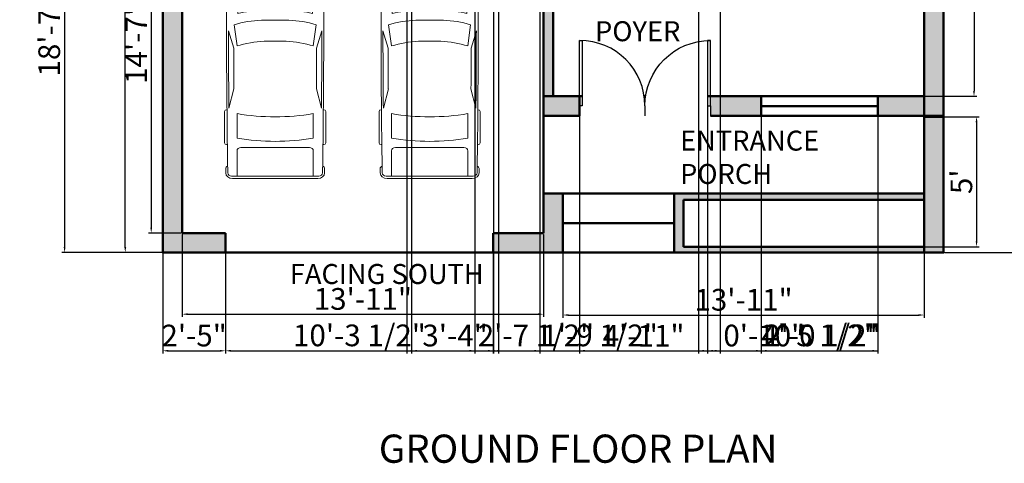
# Model space of a CAD drawing. Units: inches. Extents: x 1344 to 2521, y 3236 to 4924.
# Tile 8 of 14: x 1348 to 1801, y 4056 to 4260. Entities that reach past the tile are written whole.
import ezdxf

# ---------------------------------------------------------------- set-up
doc = ezdxf.new("R2010")
doc.units = ezdxf.units.IN
for name, color, linetype, lineweight in [('A-ANNO-DIMS', 2, 'Continuous', 18), ('A-ANNO-TEXT', 7, 'Continuous', 25), ('A-AREA-IDEN', 3, 'Continuous', 18), ('A-DOOR', 50, 'Continuous', 25), ('A-WALL', 31, 'Continuous', 50), ('A-WALL-PATT', 8, 'Continuous', 13), ('C-PKNG', 193, 'Continuous', 18)]:
    doc.layers.add(name, color=color, linetype=linetype, lineweight=lineweight)
doc.styles.get("Standard").update_dxf_attribs({"font": 'arial.ttf'})
doc.dimstyles.new('ISO-25', dxfattribs={"dimtxt": 10, "dimasz": 2.5, "dimexe": 1.25, "dimexo": 0.625, "dimtad": 1, "dimdec": 0, "dimlunit": 4, "dimtxsty": 'Standard', "dimcen": 2.5, "dimadec": 0, "dimazin": 0, "dimtfac": 1, "dimtdec": 0, "dimtmove": 0, "dimatfit": 3, "dimfxl": 1, "dimarcsym": 0})

# ---------------------------------------------------------------- blocks, each defined once
blk = doc.blocks.new('*U4')
for p, q in [((46.55, 38.89), (22.35, 38.89)), ((136.7, 38.89), (160.9, 38.89)), ((21.1, 37.41), (21.1, 36.83)), ((47.8, 37.39), (47.8, 37.41)), ((70.03, 31.54), (86.41, 29.35)), ((87.99, 31.87), (74.76, 35.92)), ((134.31, 35.6), (119.29, 31.78)), ((135.45, 37.07), (135.45, 37.41)), ((162.15, 37.41), (162.15, 36.77)), ((186.47, -33.5), (186.47, 33.5)), ((188.4, -32.76), (188.4, 32.76)), ((138.42, 29.35), (157.25, 29.35)), ((164.52, 26.39), (164.52, -26.39)), ((186.47, 29.35), (167.01, 29.35)), ((32.27, 11.63), (36.13, 17.17)), ((36.13, 17.17), (50.94, 17.17)), ((29.77, 9.51), (51.68, 9.51)), ((32.12, 9.51), (32.12, 11.15)), ((58.92, -10.77), (58.92, 10.77)), ((66.55, -10.53), (66.55, 10.53)), ((82.74, 8.5), (82.74, -8.5)), ((186.47, -10.53), (186.47, 10.53)), ((3.27, 6.13), (0.1, 0.41)), ((0, 0), (51.68, 0)), ((0.1, -0.41), (3.27, -6.13)), ((29.77, -9.51), (51.68, -9.51)), ((32.12, -9.51), (32.12, -11.15)), ((32.27, -11.63), (36.13, -17.17)), ((36.13, -17.17), (50.94, -17.17)), ((86.41, -29.35), (70.03, -31.54)), ((157.25, -29.35), (138.42, -29.35)), ((167.01, -29.35), (186.47, -29.35)), ((21.1, -37.41), (21.1, -36.83)), ((47.8, -37.39), (47.8, -37.41)), ((87.99, -31.87), (74.76, -35.92)), ((134.31, -35.6), (119.29, -31.78)), ((135.45, -37.07), (135.45, -37.41)), ((162.15, -37.41), (162.15, -36.77)), ((46.55, -38.89), (22.35, -38.89)), ((136.7, -38.89), (160.9, -38.89))]:
    blk.add_line(p, q)
for centre, major_axis, ratio, start_param, end_param in [((22.35, 37.41), (0, -1.48), 0.842304, 3.141593, 4.712389), ((46.55, 37.41), (0, 1.48), 0.842304, -1.570796, 0), ((136.7, 37.41), (0, -1.48), 0.842304, 3.141593, 4.712389), ((160.9, 37.41), (0, 1.48), 0.842304, -1.570796, 0), ((180.63, 35.84), (0, 2.22), 0.842304, -0.013017, 1.249894), ((64.48, -10556.36), (0, 10595.31), 0.842304, -0.013397, -0.013017), ((183.98, 32.76), (0, -5.25), 0.842304, 1.570796, 3.128196), ((266.03, -27.52), (0, 313.31), 0.842304, 1.367076, 1.39176), ((41.19, -490.86), (0, 528.23), 0.842304, 0.00281, 0.075598), ((64.48, -10555.62), (0, 10593.03), 0.842304, -0.013397, 0.002797), ((135.29, 5.39), (0, 81.77), 0.842304, 1.245306, 1.50788), ((64.48, -10555.62), (0, -10591.55), 0.842304, 3.133765, 3.140441), ((95.79, -3666.35), (0, -3698.24), 0.842304, 3.134049, 3.144098), ((183.98, 33.5), (0, -2.96), 0.842304, 1.570796, 3.128196), ((259.18, -27.52), (0, -305.3), 0.842304, 4.528606, 4.561838), ((37.47, -593.96), (0, -623.33), 0.842304, 3.096046, 3.200911), ((134.4, 5.39), (0, -89.78), 0.842304, 4.449482, 4.652344), ((149.6, 2.8), (0, -79.58), 0.842304, 4.372215, 4.640744), ((17.08, 0), (0, 147.02), 0.842304, 4.511394, 4.913384), ((35.91, 0), (0, 147.02), 0.842304, 4.511394, 4.913384), ((167.01, 26.39), (0, 2.96), 0.842304, 0, 1.570796), ((-204.49, 52.4), (0, -250.96), 0.842304, 1.385369, 1.434372), ((13.04, 17.01), (0, 27.42), 0.842304, 4.435146, 4.718221), ((14.2, 17.01), (0, 27.42), 0.842304, 4.435146, 4.718221), ((50.79, 13.34), (6.34, -0.36), 0.603834, -1.395552, 1.581315), ((29.77, -46.66), (0, 56.17), 0.842304, 0, 0.590319), ((32.75, 11.15), (0, 0.74), 0.842304, 0.879714, 1.570796), ((0.62, 0), (0, -0.74), 0.842304, 4.131459, 5.293319), ((-204.49, -52.4), (0, 250.96), 0.842304, -1.434372, -1.385369), ((29.77, 46.66), (0, 56.17), 0.842304, 2.551274, 3.141593), ((32.75, -11.15), (0, -0.74), 0.842304, 4.712389, 5.403472), ((13.04, -17.01), (0, -27.42), 0.842304, 1.564964, 1.848039), ((14.2, -17.01), (0, -27.42), 0.842304, 1.564964, 1.848039), ((134.4, -5.39), (0, -89.78), 0.842304, -1.510751, -1.307889), ((135.29, -5.39), (0, -81.77), 0.842304, -1.50788, -1.245306), ((149.6, -2.8), (0, -79.58), 0.842304, -1.499151, -1.230623), ((259.18, 27.52), (0, 305.3), 0.842304, 1.721348, 1.754579), ((266.03, 27.52), (0, 313.31), 0.842304, 1.749832, 1.774517), ((37.47, 593.96), (0, -623.33), 0.842304, -0.059319, 0.045547), ((167.01, -26.39), (0, -2.96), 0.842304, 4.712389, 6.283185), ((41.19, 490.86), (0, -528.23), 0.842304, -0.075598, -0.00281), ((22.35, -37.41), (0, 1.48), 0.842304, 1.570796, 3.141593), ((64.48, 10555.62), (0, 10593.03), 0.842304, 3.138796, 3.15499), ((46.55, -37.41), (0, -1.48), 0.842304, 0, 1.570796), ((64.48, 10555.62), (0, -10591.55), 0.842304, 0.001152, 0.007828), ((95.79, 3666.35), (0, -3698.24), 0.842304, -0.002505, 0.007544), ((136.7, -37.41), (0, -1.48), 0.842304, -1.570796, 0), ((160.9, -37.41), (0, 1.48), 0.842304, 3.141593, 4.712389), ((180.63, -35.84), (0, -2.22), 0.842304, -1.249894, 0.013017), ((183.98, -33.5), (0, 2.96), 0.842304, 3.15499, 4.712389), ((183.98, -32.76), (0, -5.25), 0.842304, 0.013397, 1.570796), ((64.48, 10556.36), (0, 10595.31), 0.842304, 3.15461, 3.15499)]:
    blk.add_ellipse(centre, major_axis=major_axis, ratio=ratio, start_param=start_param, end_param=end_param)
at = {"extrusion": (0, 0, -1)}
blk.add_ellipse((50.79, -13.34), major_axis=(6.34, 0.36), ratio=0.603834, start_param=-1.395552, end_param=1.581315, dxfattribs=at)
blk = doc.blocks.new('*U2')
for p, q in [((0, 0), (0, -6)), ((40, 0), (40, -6))]:
    blk.add_line(p, q)
blk.add_lwpolyline([(0, 0), (0, 40), (1.75, 40), (1.75, 0)], close=True)
blk.add_arc((0, 0), 40, 0, 90)
blk = doc.blocks.new('*D16')
at = {"layer": 'A-ANNO-DIMS', "color": 0, "lineweight": -2, "transparency": 16777216}
for p, q in [((1412.89, 4753.21), (1394.98, 4753.21)), ((1396.23, 4155.71), (1396.23, 4750.71)), ((1412.89, 4153.21), (1394.98, 4153.21))]:
    blk.add_line(p, q, dxfattribs=at)
at = {"layer": 'A-ANNO-DIMS', "color": 0, "lineweight": 100, "transparency": 16777216}
for points in [[(1395.81, 4750.71), (1396.65, 4750.71), (1396.23, 4753.21)], [(1395.81, 4155.71), (1396.65, 4155.71), (1396.23, 4153.21)]]:
    blk.add_solid(points, dxfattribs=at)
at = {"layer": 'Defpoints', "color": 0, "lineweight": 100, "transparency": 16777216}
for p in [(1396.23, 4753.21), (1413.52, 4753.21), (1413.52, 4153.21)]:
    blk.add_point(p, dxfattribs=at)
at = {"layer": 'A-ANNO-DIMS', "color": 0, "transparency": 16777216, "insert": (1390.5, 4453.21), "char_height": 10, "attachment_point": 5, "rotation": 90}
blk.add_mtext("50'", dxfattribs=at)
blk = doc.blocks.new('*D24')
at = {"layer": 'A-ANNO-DIMS', "color": 0, "lineweight": -2, "transparency": 16777216}
for p, q in [((1421.89, 4337.29), (1406.95, 4337.29)), ((1408.2, 4334.79), (1408.2, 4164.71)), ((1421.89, 4162.21), (1406.95, 4162.21))]:
    blk.add_line(p, q, dxfattribs=at)
at = {"layer": 'A-ANNO-DIMS', "color": 0, "lineweight": 100, "transparency": 16777216}
for points in [[(1407.78, 4334.79), (1408.61, 4334.79), (1408.2, 4337.29)], [(1407.78, 4164.71), (1408.61, 4164.71), (1408.2, 4162.21)]]:
    blk.add_solid(points, dxfattribs=at)
at = {"layer": 'Defpoints', "color": 0, "lineweight": 100, "transparency": 16777216}
for p in [(1422.52, 4337.29), (1408.2, 4162.21), (1422.52, 4162.21)]:
    blk.add_point(p, dxfattribs=at)
at = {"layer": 'A-ANNO-DIMS', "color": 0, "transparency": 16777216, "insert": (1402.55, 4249.75), "char_height": 10, "attachment_point": 5, "rotation": 90}
blk.add_mtext('14\'-7"', dxfattribs=at)
blk = doc.blocks.new('*D25')
at = {"layer": 'A-ANNO-DIMS', "color": 0, "lineweight": -2, "transparency": 16777216}
for p, q in [((1422.52, 4161.59), (1422.52, 4123.57)), ((1589.02, 4161.59), (1589.02, 4123.57)), ((1425.02, 4124.82), (1586.52, 4124.82))]:
    blk.add_line(p, q, dxfattribs=at)
at = {"layer": 'A-ANNO-DIMS', "color": 0, "lineweight": 100, "transparency": 16777216}
for points in [[(1425.02, 4125.24), (1425.02, 4124.41), (1422.52, 4124.82)], [(1586.52, 4125.24), (1586.52, 4124.41), (1589.02, 4124.82)]]:
    blk.add_solid(points, dxfattribs=at)
at = {"layer": 'Defpoints', "color": 0, "lineweight": 100, "transparency": 16777216}
for p in [(1422.52, 4162.21), (1589.02, 4162.21), (1589.02, 4124.82)]:
    blk.add_point(p, dxfattribs=at)
at = {"layer": 'A-ANNO-DIMS', "color": 0, "transparency": 16777216, "insert": (1505.77, 4130.56), "char_height": 10, "attachment_point": 5}
blk.add_mtext('13\'-11"', dxfattribs=at)
blk = doc.blocks.new('*D26')
at = {"layer": 'A-ANNO-DIMS', "color": 0, "lineweight": -2, "transparency": 16777216}
for p, q in [((1764.52, 4155.25), (1764.52, 4123.19)), ((1598.02, 4152.59), (1598.02, 4123.19)), ((1600.52, 4124.44), (1762.02, 4124.44))]:
    blk.add_line(p, q, dxfattribs=at)
at = {"layer": 'A-ANNO-DIMS', "color": 0, "lineweight": 100, "transparency": 16777216}
for points in [[(1600.52, 4124.85), (1600.52, 4124.02), (1598.02, 4124.44)], [(1762.02, 4124.85), (1762.02, 4124.02), (1764.52, 4124.44)]]:
    blk.add_solid(points, dxfattribs=at)
at = {"layer": 'Defpoints', "color": 0, "lineweight": 100, "transparency": 16777216}
for p in [(1764.52, 4155.88), (1598.02, 4153.21), (1764.52, 4124.44)]:
    blk.add_point(p, dxfattribs=at)
at = {"layer": 'A-ANNO-DIMS', "color": 0, "transparency": 16777216, "insert": (1681.27, 4130.17), "char_height": 10, "attachment_point": 5}
blk.add_mtext('13\'-11"', dxfattribs=at)
blk = doc.blocks.new('*D27')
at = {"layer": 'A-ANNO-DIMS', "color": 0, "lineweight": -2, "transparency": 16777216}
for p, q in [((1765.14, 4215.79), (1789.95, 4215.79)), ((1788.7, 4213.29), (1788.7, 4158.38)), ((1765.14, 4155.88), (1789.95, 4155.88))]:
    blk.add_line(p, q, dxfattribs=at)
at = {"layer": 'A-ANNO-DIMS', "color": 0, "lineweight": 100, "transparency": 16777216}
for points in [[(1788.28, 4213.29), (1789.12, 4213.29), (1788.7, 4215.79)], [(1788.28, 4158.38), (1789.12, 4158.38), (1788.7, 4155.88)]]:
    blk.add_solid(points, dxfattribs=at)
at = {"layer": 'Defpoints', "color": 0, "lineweight": 100, "transparency": 16777216}
for p in [(1764.52, 4215.79), (1764.52, 4155.88), (1788.7, 4155.88)]:
    blk.add_point(p, dxfattribs=at)
at = {"layer": 'A-ANNO-DIMS', "color": 0, "transparency": 16777216, "insert": (1782.99, 4185.84), "char_height": 10, "attachment_point": 5, "rotation": 90}
blk.add_mtext("5'", dxfattribs=at)
blk = doc.blocks.new('*D28')
at = {"layer": 'A-ANNO-DIMS', "color": 0, "lineweight": -2, "transparency": 16777216}
for p, q in [((1765.14, 4382.64), (1788.78, 4382.64)), ((1787.53, 4380.14), (1787.53, 4227.72)), ((1765.14, 4225.22), (1788.78, 4225.22))]:
    blk.add_line(p, q, dxfattribs=at)
at = {"layer": 'A-ANNO-DIMS', "color": 0, "lineweight": 100, "transparency": 16777216}
for points in [[(1787.11, 4380.14), (1787.95, 4380.14), (1787.53, 4382.64)], [(1787.11, 4227.72), (1787.95, 4227.72), (1787.53, 4225.22)]]:
    blk.add_solid(points, dxfattribs=at)
at = {"layer": 'Defpoints', "color": 0, "lineweight": 100, "transparency": 16777216}
for p in [(1764.52, 4382.64), (1764.52, 4225.22), (1787.53, 4225.22)]:
    blk.add_point(p, dxfattribs=at)
at = {"layer": 'A-ANNO-DIMS', "color": 0, "transparency": 16777216, "insert": (1781.8, 4303.93), "char_height": 10, "attachment_point": 5, "rotation": 90}
blk.add_mtext('13\'-1"', dxfattribs=at)
blk = doc.blocks.new('*D84')
at = {"layer": 'A-ANNO-DIMS', "color": 0, "lineweight": -2, "transparency": 16777216}
for p, q in [((1412.89, 4376.68), (1367.02, 4376.68)), ((1368.27, 4374.18), (1368.27, 4155.71)), ((1412.89, 4153.21), (1367.02, 4153.21))]:
    blk.add_line(p, q, dxfattribs=at)
at = {"layer": 'A-ANNO-DIMS', "color": 0, "lineweight": 100, "transparency": 16777216}
for points in [[(1367.85, 4374.18), (1368.68, 4374.18), (1368.27, 4376.68)], [(1367.85, 4155.71), (1368.68, 4155.71), (1368.27, 4153.21)]]:
    blk.add_solid(points, dxfattribs=at)
at = {"layer": 'Defpoints', "color": 0, "lineweight": 100, "transparency": 16777216}
for p in [(1413.52, 4376.68), (1368.27, 4153.21), (1413.52, 4153.21)]:
    blk.add_point(p, dxfattribs=at)
at = {"layer": 'A-ANNO-DIMS', "color": 0, "transparency": 16777216, "insert": (1362.47, 4264.94), "char_height": 10, "attachment_point": 5, "rotation": 90}
blk.add_mtext('18\'-7 1/2"', dxfattribs=at)
blk = doc.blocks.new('*D89')
at = {"layer": 'A-ANNO-DIMS', "color": 0, "lineweight": -2, "transparency": 16777216}
for p, q in [((1774.14, 4425.27), (1820.02, 4425.27)), ((1818.77, 4422.77), (1818.77, 4155.71)), ((1774.14, 4153.21), (1820.02, 4153.21))]:
    blk.add_line(p, q, dxfattribs=at)
at = {"layer": 'A-ANNO-DIMS', "color": 0, "lineweight": 100, "transparency": 16777216}
for points in [[(1818.35, 4422.77), (1819.18, 4422.77), (1818.77, 4425.27)], [(1818.35, 4155.71), (1819.18, 4155.71), (1818.77, 4153.21)]]:
    blk.add_solid(points, dxfattribs=at)
at = {"layer": 'Defpoints', "color": 0, "lineweight": 100, "transparency": 16777216}
for p in [(1773.52, 4425.27), (1773.52, 4153.21), (1818.77, 4153.21)]:
    blk.add_point(p, dxfattribs=at)
at = {"layer": 'A-ANNO-DIMS', "color": 0, "transparency": 16777216, "insert": (1813.04, 4289.24), "char_height": 10, "attachment_point": 5, "rotation": 90}
blk.add_mtext('22\'-8"', dxfattribs=at)
blk = doc.blocks.new('*D90')
at = {"layer": 'A-ANNO-DIMS', "color": 0, "lineweight": -2, "transparency": 16777216}
for p, q in [((1413.52, 4152.59), (1413.52, 4106.71)), ((1442.43, 4152.59), (1442.43, 4106.71)), ((1416.02, 4107.96), (1439.93, 4107.96))]:
    blk.add_line(p, q, dxfattribs=at)
at = {"layer": 'A-ANNO-DIMS', "color": 0, "lineweight": 100, "transparency": 16777216}
for points in [[(1416.02, 4108.38), (1416.02, 4107.54), (1413.52, 4107.96)], [(1439.93, 4108.38), (1439.93, 4107.54), (1442.43, 4107.96)]]:
    blk.add_solid(points, dxfattribs=at)
at = {"layer": 'Defpoints', "color": 0, "lineweight": 100, "transparency": 16777216}
for p in [(1413.52, 4153.21), (1442.43, 4153.21), (1442.43, 4107.96)]:
    blk.add_point(p, dxfattribs=at)
at = {"layer": 'A-ANNO-DIMS', "color": 0, "transparency": 16777216, "insert": (1427.97, 4113.69), "char_height": 10, "attachment_point": 5}
blk.add_mtext('2\'-5"', dxfattribs=at)
blk = doc.blocks.new('*D91')
at = {"layer": 'A-ANNO-DIMS', "color": 0, "lineweight": -2, "transparency": 16777216}
for p, q in [((1442.43, 4152.59), (1442.43, 4106.71)), ((1565.92, 4152.59), (1565.92, 4106.71)), ((1444.93, 4107.96), (1563.42, 4107.96))]:
    blk.add_line(p, q, dxfattribs=at)
at = {"layer": 'A-ANNO-DIMS', "color": 0, "lineweight": 100, "transparency": 16777216}
for points in [[(1444.93, 4108.38), (1444.93, 4107.54), (1442.43, 4107.96)], [(1563.42, 4108.38), (1563.42, 4107.54), (1565.92, 4107.96)]]:
    blk.add_solid(points, dxfattribs=at)
at = {"layer": 'Defpoints', "color": 0, "lineweight": 100, "transparency": 16777216}
for p in [(1442.43, 4153.21), (1565.92, 4153.21), (1565.92, 4107.96)]:
    blk.add_point(p, dxfattribs=at)
at = {"layer": 'A-ANNO-DIMS', "color": 0, "transparency": 16777216, "insert": (1504.18, 4113.76), "char_height": 10, "attachment_point": 5}
blk.add_mtext('10\'-3 1/2"', dxfattribs=at)
blk = doc.blocks.new('*D93')
at = {"layer": 'A-ANNO-DIMS', "color": 0, "lineweight": -2, "transparency": 16777216}
for p, q in [((1526.04, 4667.09), (1526.04, 4106.71)), ((1557.42, 4667.09), (1557.42, 4106.71)), ((1528.54, 4107.96), (1554.92, 4107.96)), ((1557.42, 4107.96), (1611.23, 4107.96))]:
    blk.add_line(p, q, dxfattribs=at)
at = {"layer": 'A-ANNO-DIMS', "color": 0, "lineweight": 100, "transparency": 16777216}
for points in [[(1528.54, 4108.38), (1528.54, 4107.54), (1526.04, 4107.96)], [(1554.92, 4108.38), (1554.92, 4107.54), (1557.42, 4107.96)]]:
    blk.add_solid(points, dxfattribs=at)
at = {"layer": 'Defpoints', "color": 0, "lineweight": 100, "transparency": 16777216}
for p in [(1526.04, 4667.71), (1557.42, 4667.71), (1557.42, 4107.96)]:
    blk.add_point(p, dxfattribs=at)
at = {"layer": 'A-ANNO-DIMS', "color": 0, "transparency": 16777216, "insert": (1585.57, 4113.76), "char_height": 10, "attachment_point": 5}
blk.add_mtext('2\'-7 1/2"', dxfattribs=at)
blk = doc.blocks.new('*D95')
at = {"layer": 'A-ANNO-DIMS', "color": 0, "lineweight": -2, "transparency": 16777216}
for p, q in [((1528.27, 4522.42), (1528.27, 4106.71)), ((1568.27, 4522.42), (1568.27, 4106.71)), ((1530.77, 4107.96), (1565.77, 4107.96))]:
    blk.add_line(p, q, dxfattribs=at)
at = {"layer": 'A-ANNO-DIMS', "color": 0, "lineweight": 100, "transparency": 16777216}
for points in [[(1530.77, 4108.38), (1530.77, 4107.54), (1528.27, 4107.96)], [(1565.77, 4108.38), (1565.77, 4107.54), (1568.27, 4107.96)]]:
    blk.add_solid(points, dxfattribs=at)
at = {"layer": 'Defpoints', "color": 0, "lineweight": 100, "transparency": 16777216}
for p in [(1528.27, 4523.04), (1568.27, 4523.04), (1568.27, 4107.96)]:
    blk.add_point(p, dxfattribs=at)
at = {"layer": 'A-ANNO-DIMS', "color": 0, "transparency": 16777216, "insert": (1548.27, 4113.7), "char_height": 10, "attachment_point": 5}
blk.add_mtext('3\'-4"', dxfattribs=at)
blk = doc.blocks.new('*D97')
at = {"layer": 'A-ANNO-DIMS', "color": 0, "lineweight": -2, "transparency": 16777216}
for p, q in [((1566.07, 4465.94), (1566.07, 4106.71)), ((1587.33, 4458.96), (1587.33, 4106.71)), ((1568.57, 4107.96), (1584.83, 4107.96)), ((1587.33, 4107.96), (1640.02, 4107.96))]:
    blk.add_line(p, q, dxfattribs=at)
at = {"layer": 'A-ANNO-DIMS', "color": 0, "lineweight": 100, "transparency": 16777216}
for points in [[(1568.57, 4108.38), (1568.57, 4107.54), (1566.07, 4107.96)], [(1584.83, 4108.38), (1584.83, 4107.54), (1587.33, 4107.96)]]:
    blk.add_solid(points, dxfattribs=at)
at = {"layer": 'Defpoints', "color": 0, "lineweight": 100, "transparency": 16777216}
for p in [(1566.07, 4466.57), (1587.33, 4459.59), (1587.33, 4107.96)]:
    blk.add_point(p, dxfattribs=at)
at = {"layer": 'A-ANNO-DIMS', "color": 0, "transparency": 16777216, "insert": (1614.92, 4113.76), "char_height": 10, "attachment_point": 5}
blk.add_mtext('1\'-9 1/2"', dxfattribs=at)
blk = doc.blocks.new('*D100')
at = {"layer": 'A-ANNO-DIMS', "color": 0, "lineweight": -2, "transparency": 16777216}
for p, q in [((1660.52, 4522.42), (1660.52, 4106.71)), ((1670.52, 4522.42), (1670.52, 4106.71)), ((1663.02, 4107.96), (1668.02, 4107.96)), ((1670.52, 4107.96), (1708.62, 4107.96))]:
    blk.add_line(p, q, dxfattribs=at)
at = {"layer": 'A-ANNO-DIMS', "color": 0, "lineweight": 100, "transparency": 16777216}
for points in [[(1663.02, 4108.38), (1663.02, 4107.54), (1660.52, 4107.96)], [(1668.02, 4108.38), (1668.02, 4107.54), (1670.52, 4107.96)]]:
    blk.add_solid(points, dxfattribs=at)
at = {"layer": 'Defpoints', "color": 0, "lineweight": 100, "transparency": 16777216}
for p in [(1660.52, 4523.04), (1670.52, 4523.04), (1670.52, 4107.96)]:
    blk.add_point(p, dxfattribs=at)
at = {"layer": 'A-ANNO-DIMS', "color": 0, "transparency": 16777216, "insert": (1690.82, 4113.69), "char_height": 10, "attachment_point": 5}
blk.add_mtext('0\'-10"', dxfattribs=at)
blk = doc.blocks.new('*D106')
at = {"layer": 'A-ANNO-DIMS', "color": 0, "lineweight": -2, "transparency": 16777216}
for p, q in [((1605.63, 4224.59), (1605.63, 4106.71)), ((1664.72, 4224.59), (1664.72, 4106.71)), ((1608.13, 4107.96), (1662.22, 4107.96))]:
    blk.add_line(p, q, dxfattribs=at)
at = {"layer": 'A-ANNO-DIMS', "color": 0, "lineweight": 100, "transparency": 16777216}
for points in [[(1608.13, 4108.38), (1608.13, 4107.54), (1605.63, 4107.96)], [(1662.22, 4108.38), (1662.22, 4107.54), (1664.72, 4107.96)]]:
    blk.add_solid(points, dxfattribs=at)
at = {"layer": 'Defpoints', "color": 0, "lineweight": 100, "transparency": 16777216}
for p in [(1605.63, 4225.22), (1664.72, 4225.22), (1664.72, 4107.96)]:
    blk.add_point(p, dxfattribs=at)
at = {"layer": 'A-ANNO-DIMS', "color": 0, "transparency": 16777216, "insert": (1635.18, 4113.61), "char_height": 10, "attachment_point": 5}
blk.add_mtext('4\'-11"', dxfattribs=at)
blk = doc.blocks.new('*D107')
at = {"layer": 'A-ANNO-DIMS', "color": 0, "lineweight": -2, "transparency": 16777216}
for p, q in [((1664.72, 4224.59), (1664.72, 4106.71)), ((1689.47, 4224.59), (1689.47, 4106.71)), ((1667.22, 4107.96), (1686.97, 4107.96)), ((1689.47, 4107.96), (1743.28, 4107.96))]:
    blk.add_line(p, q, dxfattribs=at)
at = {"layer": 'A-ANNO-DIMS', "color": 0, "lineweight": 100, "transparency": 16777216}
for points in [[(1667.22, 4108.38), (1667.22, 4107.54), (1664.72, 4107.96)], [(1686.97, 4108.38), (1686.97, 4107.54), (1689.47, 4107.96)]]:
    blk.add_solid(points, dxfattribs=at)
at = {"layer": 'Defpoints', "color": 0, "lineweight": 100, "transparency": 16777216}
for p in [(1664.72, 4225.22), (1689.47, 4225.22), (1689.47, 4107.96)]:
    blk.add_point(p, dxfattribs=at)
at = {"layer": 'A-ANNO-DIMS', "color": 0, "transparency": 16777216, "insert": (1717.62, 4113.76), "char_height": 10, "attachment_point": 5}
blk.add_mtext('2\'-0 1/2"', dxfattribs=at)
blk = doc.blocks.new('*D108')
at = {"layer": 'A-ANNO-DIMS', "color": 0, "lineweight": -2, "transparency": 16777216}
for p, q in [((1689.47, 4224.59), (1689.47, 4106.71)), ((1743.16, 4224.59), (1743.16, 4106.71)), ((1691.97, 4107.96), (1740.66, 4107.96))]:
    blk.add_line(p, q, dxfattribs=at)
at = {"layer": 'A-ANNO-DIMS', "color": 0, "lineweight": 100, "transparency": 16777216}
for points in [[(1691.97, 4108.38), (1691.97, 4107.54), (1689.47, 4107.96)], [(1740.66, 4108.38), (1740.66, 4107.54), (1743.16, 4107.96)]]:
    blk.add_solid(points, dxfattribs=at)
at = {"layer": 'Defpoints', "color": 0, "lineweight": 100, "transparency": 16777216}
for p in [(1689.47, 4225.22), (1743.16, 4225.22), (1743.16, 4107.96)]:
    blk.add_point(p, dxfattribs=at)
at = {"layer": 'A-ANNO-DIMS', "color": 0, "transparency": 16777216, "insert": (1716.32, 4113.76), "char_height": 10, "attachment_point": 5}
blk.add_mtext('4\'-5 1/2"', dxfattribs=at)

msp = doc.modelspace()

# ---------------------------------------------------------------- hatches: boundary and pattern name
at = {"layer": 'A-WALL-PATT'}
h = msp.add_hatch(color=256, dxfattribs=at)
h.dxf.hatch_style = 1
h.paths.add_polyline_path([(1773.52, 4425.27), (1764.52, 4425.27), (1764.52, 4225.22), (1743.16, 4225.22), (1743.16, 4216.22), (1764.52, 4216.22), (1764.52, 4162.21), (1764.52, 4155.88), (1653.6, 4155.88), (1653.6, 4177.58), (1764.52, 4177.58), (1764.52, 4180.4), (1649.25, 4180.4), (1649.25, 4153.21), (1773.52, 4153.21)], flags=17)
h.paths.add_polyline_path([(1598.02, 4180.38), (1593.52, 4180.38), (1589.02, 4180.38), (1589.02, 4162.21), (1565.92, 4162.21), (1565.92, 4153.21), (1598.02, 4153.21)], flags=17)
h.paths.add_polyline_path([(1689.47, 4225.22), (1666.04, 4225.22), (1666.04, 4220.75), (1666.04, 4216.22), (1689.47, 4216.22)], flags=16)
h.paths.add_polyline_path([(1442.43, 4162.21), (1422.52, 4162.21), (1422.52, 4744.21), (1764.52, 4744.21), (1764.52, 4225.22), (1743.16, 4225.22), (1743.16, 4216.22), (1764.52, 4216.22), (1764.52, 4162.21), (1764.52, 4155.88), (1653.6, 4155.88), (1653.6, 4177.58), (1764.52, 4177.58), (1764.52, 4180.4), (1649.25, 4180.4), (1649.25, 4153.21), (1773.52, 4153.21), (1773.52, 4425.27), (1773.52, 4753.21), (1413.52, 4753.21), (1413.52, 4153.21), (1442.43, 4153.21)])
h.paths.add_polyline_path([(1648.69, 4179.48), (1724.08, 4179.48), (1724.08, 4213.98), (1648.69, 4213.98)], flags=25)
h.paths.add_polyline_path([(1609.51, 4245.39), (1659.17, 4245.39), (1659.17, 4264.37), (1609.51, 4264.37)], flags=25)
h.paths.add_polyline_path([(1618.52, 4270.74), (1667.67, 4270.74), (1667.67, 4305.24), (1618.52, 4305.24)], flags=25)
h.paths.add_polyline_path([(1563.46, 4499.55), (1651.73, 4499.55), (1651.73, 4518.53), (1563.46, 4518.53)], flags=25)
h.paths.add_polyline_path([(1439.72, 4433.21), (1521.54, 4433.21), (1521.54, 4467.71), (1439.72, 4467.71)], flags=25)
h.paths.add_polyline_path([(1651.43, 4581.89), (1735.04, 4581.89), (1735.04, 4616.38), (1651.43, 4616.38)], flags=25)
h.paths.add_polyline_path([(1495.42, 4585.56), (1566.53, 4585.56), (1566.53, 4620.06), (1495.42, 4620.06)], flags=25)
h.paths.add_polyline_path([(1677.05, 4699.47), (1729.56, 4699.47), (1729.56, 4718.45), (1677.05, 4718.45)], flags=25)
h.paths.add_polyline_path([(1581.37, 4669.39), (1626.01, 4669.39), (1626.01, 4703.88), (1581.37, 4703.88)], flags=25)
h.paths.add_polyline_path([(1523.21, 4717.23), (1572.85, 4717.23), (1572.85, 4736.21), (1523.21, 4736.21)], flags=25)
h.paths.add_polyline_path([(1432.59, 4685.86), (1482.24, 4685.86), (1482.24, 4704.84), (1432.59, 4704.84)], flags=25)
h = msp.add_hatch(color=256, dxfattribs=at)
h.dxf.hatch_style = 1
h.paths.add_polyline_path([(1773.52, 4215.79), (1764.52, 4215.79), (1764.52, 4153.21), (1773.52, 4153.21)])
h.paths.add_polyline_path([(1773.52, 4425.27), (1764.52, 4425.27), (1764.52, 4216.22), (1773.52, 4216.22)])
h.paths.add_polyline_path([(1764.52, 4225.22), (1743.16, 4225.22), (1743.16, 4216.22), (1764.52, 4216.22)])
h.paths.add_polyline_path([(1764.52, 4180.4), (1649.25, 4180.4), (1649.25, 4153.21), (1764.52, 4153.21), (1764.52, 4155.88), (1653.6, 4155.88), (1653.6, 4177.58), (1764.52, 4177.58)])
h.paths.add_polyline_path([(1605.63, 4225.22), (1589.02, 4225.22), (1589.02, 4216.22), (1605.63, 4216.22)])
h.paths.add_polyline_path([(1593.52, 4382.64), (1589.02, 4382.64), (1589.02, 4225.22), (1593.52, 4225.22)])
h.paths.add_polyline_path([(1544.94, 4341.79), (1422.52, 4341.79), (1422.52, 4337.29), (1544.94, 4337.29)])
h.paths.add_polyline_path([(1593.52, 4387.14), (1561.57, 4387.14), (1561.57, 4382.64), (1593.52, 4382.64)])
h.paths.add_polyline_path([(1566.07, 4466.57), (1561.57, 4466.57), (1561.57, 4387.14), (1566.07, 4387.14)])

# ---------------------------------------------------------------- linework, layer by layer
at = {"layer": 'A-WALL'}
for p, q in [((1589.02, 4162.21), (1589.02, 4382.64)), ((1593.52, 4225.22), (1593.52, 4382.64)), ((1606.95, 4225.22), (1593.52, 4225.22)), ((1636.17, 4225.22), (1635.51, 4225.22)), ((1764.52, 4225.22), (1664.72, 4225.22)), ((1689.47, 4220.72), (1743.16, 4220.72)), ((1593.52, 4216.22), (1589.02, 4216.22)), ((1605.63, 4216.22), (1593.52, 4216.22)), ((1764.52, 4216.22), (1666.04, 4216.22)), ((1593.52, 4180.38), (1589.02, 4180.38)), ((1593.52, 4180.38), (1598.02, 4180.38)), ((1764.52, 4180.4), (1649.25, 4180.4)), ((1649.25, 4180.4), (1649.25, 4153.21)), ((1653.6, 4155.88), (1653.6, 4177.58)), ((1653.6, 4177.58), (1764.52, 4177.58)), ((1598.02, 4175.32), (1598.02, 4153.21)), ((1598.02, 4166.8), (1649.25, 4166.8)), ((1442.43, 4162.21), (1442.43, 4153.21)), ((1565.92, 4162.21), (1565.92, 4153.21)), ((1764.52, 4162.21), (1764.52, 4155.88)), ((1764.52, 4155.88), (1653.6, 4155.88)), ((1442.43, 4153.21), (1572.93, 4153.21))]:
    msp.add_line(p, q, dxfattribs=at)
for points in [[(1565.92, 4153.21), (1773.52, 4153.21), (1773.52, 4753.21), (1413.52, 4753.21), (1413.52, 4153.21), (1442.43, 4153.21)], [(1764.52, 4225.22), (1764.52, 4744.21), (1422.52, 4744.21), (1422.52, 4162.21), (1442.43, 4162.21)], [(1764.52, 4162.21), (1764.52, 4216.22)], [(1565.92, 4162.21), (1589.02, 4162.21)]]:
    msp.add_lwpolyline(points, dxfattribs=at)
for points in [[(1764.52, 4425.27), (1773.52, 4425.27), (1773.52, 4215.79), (1764.52, 4215.79)], [(1589.02, 4382.64), (1593.52, 4382.64), (1593.52, 4225.22), (1589.02, 4225.22)], [(1605.63, 4216.22), (1589.02, 4216.22), (1589.02, 4225.22), (1605.63, 4225.22)], [(1689.47, 4225.22), (1743.16, 4225.22), (1743.16, 4216.22), (1689.47, 4216.22)], [(1743.16, 4216.22), (1764.52, 4216.22), (1764.52, 4225.22), (1743.16, 4225.22)], [(1773.52, 4153.21), (1764.52, 4153.21), (1764.52, 4216.22), (1773.52, 4216.22)], [(1598.02, 4153.21), (1649.25, 4153.21), (1649.25, 4180.4), (1598.02, 4180.4)]]:
    msp.add_lwpolyline(points, close=True, dxfattribs=at)

# ---------------------------------------------------------------- block references
at = {"layer": 'A-DOOR', "yscale": 0.7551501978687398, "zscale": 0.7551501978687398}
for p, xscale in [((1605.63, 4220.75), 0.7551501978687398), ((1666.04, 4220.75), -0.7551501978687398)]:
    msp.add_blockref('*U2', p, dxfattribs=dict(at, xscale=xscale))
at = {"layer": 'C-PKNG', "xscale": 0.5992668008637883, "yscale": 0.5992668008637883, "zscale": 0.5992668008637883, "rotation": 270}
for p in [(1465.34, 4300.18), (1536.56, 4300.18)]:
    msp.add_blockref('*U4', p, dxfattribs=at)

# ---------------------------------------------------------------- texts
at = {"layer": 'A-ANNO-TEXT', "insert": (1513.12, 4069.35), "char_height": 12.9935, "attachment_point": 1}
msp.add_mtext_dynamic_manual_height_columns('GROUND FLOOR PLAN', width=2122.9296, gutter_width=64.97, heights=[0], dxfattribs=at)
at = {"layer": 'A-AREA-IDEN', "char_height": 9.211, "attachment_point": 1}
for s, insert in [('POYER', (1612.81, 4259.8)), ('ENTRANCE PORCH', (1652.02, 4209.39)), ('FACING SOUTH', (1472.12, 4147.94))]:
    msp.add_mtext_dynamic_manual_height_columns(s, width=108.7809, gutter_width=46.06, heights=[0], dxfattribs=dict(at, insert=insert))

# ---------------------------------------------------------------- dimensions: what is measured, and where the dimension line sits
at = {"layer": 'A-ANNO-DIMS'}
for base, p1, p2, override, picture, middle in [((1396.23, 4753.21), (1413.52, 4153.21), (1413.52, 4753.21), {"dimclrd": 0, "dimclre": 0, "dimclrt": 0}, '*D16', (1390.5, 4453.21)), ((1818.77, 4153.21), (1773.52, 4425.27), (1773.52, 4153.21), {"dimdec": 1, "dimlfac": 1, "dimrnd": 0, "dimzin": 1, "dimdsep": 46, "dimlunit": 4, "dimfrac": 2}, '*D89', (1813.04, 4289.24)), ((1787.53, 4225.22), (1764.52, 4382.64), (1764.52, 4225.22), {"dimclrd": 0, "dimclre": 0, "dimclrt": 0}, '*D28', (1781.8, 4303.93)), ((1368.27, 4153.21), (1413.52, 4376.68), (1413.52, 4153.21), {"dimdec": 1, "dimlfac": 1, "dimrnd": 0, "dimzin": 1, "dimdsep": 46, "dimlunit": 4, "dimfrac": 2}, '*D84', (1362.47, 4264.94)), ((1408.2, 4162.21), (1422.52, 4337.29), (1422.52, 4162.21), {"dimclrd": 0, "dimclre": 0, "dimclrt": 0}, '*D24', (1402.55, 4249.75)), ((1788.7, 4155.88), (1764.52, 4215.79), (1764.52, 4155.88), {"dimclrd": 0, "dimclre": 0, "dimclrt": 0}, '*D27', (1782.99, 4185.84))]:
    dim = msp.add_linear_dim(base=base, p1=p1, p2=p2, angle=90, dimstyle='ISO-25', override=override, dxfattribs=at)
    dim.commit()
    dim.dimension.update_dxf_attribs({"geometry": picture, "text_midpoint": middle})
for base, p1, p2, override, picture, middle in [((1557.42, 4107.96), (1526.04, 4667.71), (1557.42, 4667.71), {"dimdec": 1, "dimlfac": 1, "dimrnd": 0, "dimzin": 1, "dimdsep": 46, "dimlunit": 4, "dimfrac": 2}, '*D93', (1585.57, 4113.76)), ((1568.27, 4107.96), (1528.27, 4523.04), (1568.27, 4523.04), {"dimdec": 1, "dimlfac": 1, "dimrnd": 0, "dimzin": 1, "dimdsep": 46, "dimlunit": 4, "dimfrac": 2}, '*D95', (1548.27, 4113.7)), ((1670.52, 4107.96), (1660.52, 4523.04), (1670.52, 4523.04), {"dimdec": 1, "dimlfac": 1, "dimrnd": 0, "dimzin": 1, "dimdsep": 46, "dimlunit": 4, "dimfrac": 2}, '*D100', (1690.82, 4113.69)), ((1587.33, 4107.96), (1566.07, 4466.57), (1587.33, 4459.59), {"dimdec": 1, "dimlfac": 1, "dimrnd": 0, "dimzin": 1, "dimdsep": 46, "dimlunit": 4, "dimfrac": 2}, '*D97', (1614.92, 4113.76)), ((1664.72, 4107.96), (1605.63, 4225.22), (1664.72, 4225.22), {"dimdec": 1, "dimlfac": 1, "dimrnd": 0, "dimzin": 1, "dimdsep": 46, "dimlunit": 4, "dimfrac": 2}, '*D106', (1635.18, 4113.61)), ((1689.4715, 4107.9609), (1664.7228, 4225.2158), (1689.4715, 4225.2158), {"dimdec": 1, "dimlfac": 1, "dimrnd": 0, "dimzin": 1, "dimdsep": 46, "dimlunit": 4, "dimfrac": 2}, '*D107', (1717.6237, 4113.7564)), ((1743.16, 4107.96), (1689.47, 4225.22), (1743.16, 4225.22), {"dimdec": 1, "dimlfac": 1, "dimrnd": 0, "dimzin": 1, "dimdsep": 46, "dimlunit": 4, "dimfrac": 2}, '*D108', (1716.32, 4113.76)), ((1589.0178099, 4124.82382034), (1422.5178099, 4162.210881), (1589.0178099, 4162.210881), {"dimclrd": 0, "dimclre": 0, "dimclrt": 0}, '*D25', (1505.7678099, 4130.55796085)), ((1764.5178099, 4124.43693892), (1598.0178099, 4153.210881), (1764.5178099, 4155.87925272), {"dimclrd": 0, "dimclre": 0, "dimclrt": 0}, '*D26', (1681.2678099, 4130.17107944)), ((1442.43, 4107.96), (1413.52, 4153.21), (1442.43, 4153.21), {"dimdec": 1, "dimlfac": 1, "dimrnd": 0, "dimzin": 1, "dimdsep": 46, "dimlunit": 4, "dimfrac": 2}, '*D90', (1427.97, 4113.69)), ((1565.92, 4107.96), (1442.43, 4153.21), (1565.92, 4153.21), {"dimdec": 1, "dimlfac": 1, "dimrnd": 0, "dimzin": 1, "dimdsep": 46, "dimlunit": 4, "dimfrac": 2}, '*D91', (1504.18, 4113.76))]:
    dim = msp.add_linear_dim(base=base, p1=p1, p2=p2, dimstyle='ISO-25', override=override, dxfattribs=at)
    dim.commit()
    dim.dimension.update_dxf_attribs({"geometry": picture, "text_midpoint": middle})

doc.saveas('drawing.dxf')
